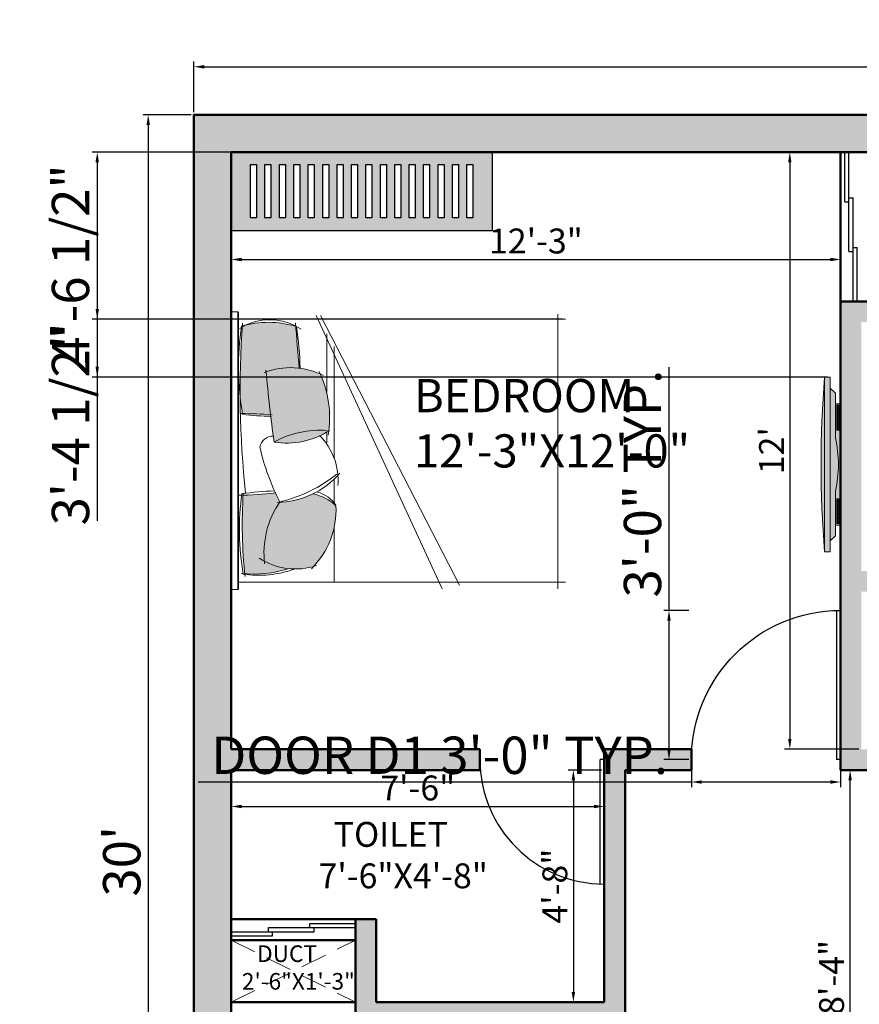
# Model space of a CAD drawing. Units: inches. Extents: x 3274 to 5176, y 1085 to 2172.
# Tile 13 of 16: x 4315 to 4518, y 1319 to 1556. Entities that reach past the tile are written whole.
import ezdxf

# ---------------------------------------------------------------- set-up
doc = ezdxf.new("R2010")
doc.units = ezdxf.units.IN
doc.linetypes.add('DASHED', pattern=[19.05, 12.7, -6.35])
for name, color, linetype, lineweight in [('0.10', 252, 'Continuous', 9), ('A-ANNO-DIMS', 2, 'Continuous', 18), ('A-AREA-IDEN', 3, 'Continuous', 25), ('A-DOOR', 4, 'Continuous', 25), ('A-EQPM', 8, 'Continuous', 18), ('A-FLOR-OPEN', 7, 'DASHED', 18), ('A-FLOR-PATT', 252, 'Continuous', 13), ('A-FURN', 8, 'Continuous', 18), ('A-GLAZ', 5, 'Continuous', 25), ('A-WALL', 7, 'Continuous', 50), ('A-WALL-PATT', 8, 'Continuous', 13), ('moveis', 254, 'Continuous', 5), ('parede', 7, 'Continuous', 30)]:
    doc.layers.add(name, color=color, linetype=linetype, lineweight=lineweight)
doc.layers.add('MESA', color=7, linetype='Continuous')
doc.styles.get("Standard").update_dxf_attribs({"font": 'arial.ttf'})
doc.dimstyles.new('ISO-25', dxfattribs={"dimtxt": 9, "dimasz": 2.5, "dimexe": 1.25, "dimexo": 0.625, "dimtad": 1, "dimdec": 1, "dimlunit": 3, "dimtxsty": 'Standard', "dimcen": 2.5, "dimclrd": 4, "dimclre": 4, "dimclrt": 1, "dimadec": 0, "dimazin": 0, "dimtfac": 1, "dimtdec": 1, "dimtmove": 0, "dimatfit": 3, "dimfxl": 1, "dimarcsym": 0})

# ---------------------------------------------------------------- blocks, each defined once
blk = doc.blocks.new('1')
for p, q in [((0, 36), (0, 0)), ((1, 36), (1, 0)), ((0, 0), (1, 0))]:
    blk.add_line(p, q)
blk.add_arc((0, 0), 36, 0, 90)
blk = doc.blocks.new('2')
for p, q in [((0, 30), (0, 0)), ((1, 30), (1, 0)), ((0, 0), (1, 0))]:
    blk.add_line(p, q)
blk.add_arc((0, 0), 30, 0, 90)
blk = doc.blocks.new('*D6')
at = {"layer": 'A-ANNO-DIMS', "color": 0, "lineweight": -2, "transparency": 16777216}
for p, q in [((4357.19, 1533.98), (4357.19, 1546.17)), ((4717.19, 1533.98), (4717.19, 1546.17)), ((4359.69, 1544.92), (4714.69, 1544.92))]:
    blk.add_line(p, q, dxfattribs=at)
at = {"layer": 'A-ANNO-DIMS', "color": 0, "transparency": 16777216}
for points in [[(4359.69, 1545.33), (4359.69, 1544.5), (4357.19, 1544.92)], [(4714.69, 1545.33), (4714.69, 1544.5), (4717.19, 1544.92)]]:
    blk.add_solid(points, dxfattribs=at)
at = {"layer": 'Defpoints', "color": 0, "transparency": 16777216}
for p in [(4717.19, 1544.92), (4357.19, 1533.35), (4717.19, 1533.35)]:
    blk.add_point(p, dxfattribs=at)
at = {"layer": 'A-ANNO-DIMS', "color": 0, "transparency": 16777216, "insert": (4537.19, 1550.14), "char_height": 9, "attachment_point": 5}
blk.add_mtext("30'", dxfattribs=at)
blk = doc.blocks.new('*D7')
at = {"layer": 'A-ANNO-DIMS', "color": 0, "lineweight": -2, "transparency": 16777216}
for p, q in [((4356.56, 1533.35), (4344.93, 1533.35)), ((4346.18, 1530.85), (4346.18, 1175.85)), ((4356.56, 1173.35), (4344.93, 1173.35))]:
    blk.add_line(p, q, dxfattribs=at)
at = {"layer": 'A-ANNO-DIMS', "color": 0, "transparency": 16777216}
for points in [[(4345.77, 1530.85), (4346.6, 1530.85), (4346.18, 1533.35)], [(4345.77, 1175.85), (4346.6, 1175.85), (4346.18, 1173.35)]]:
    blk.add_solid(points, dxfattribs=at)
at = {"layer": 'Defpoints', "color": 0, "transparency": 16777216}
for p in [(4357.19, 1533.35), (4346.18, 1173.35), (4357.19, 1173.35)]:
    blk.add_point(p, dxfattribs=at)
at = {"layer": 'A-ANNO-DIMS', "color": 0, "transparency": 16777216, "insert": (4340.96, 1353.35), "char_height": 9, "attachment_point": 5, "rotation": 90}
blk.add_mtext("30'", dxfattribs=at)
blk = doc.blocks.new('camita')
at = {"layer": '0.10'}
for p, q in [((-0.85, -0.045), (0.85, -0.045)), ((-0.805, -0.045), (-0.805, -2.0485)), ((0.805, -0.045), (0.805, -2.0485)), ((-0.8271, -0.521), (0.8464, -1.2932)), ((-0.8271, -0.5476), (0.8236, -1.3992)), ((-0.7161, -0.585), (-0.3554, -0.585)), ((-0.1136, -0.585), (-0.0485, -0.585)), ((-0.638, -0.63), (0.0434, -0.63)), ((0.1749, -0.63), (0.3179, -0.63)), ((0.4739, -0.63), (0.805, -0.63)), ((-0.8354, -2), (0.8464, -2))]:
    blk.add_line(p, q, dxfattribs=at)
blk.add_lwpolyline([(-0.85, -0.0405), (0.85, -0.0405), (0.85, 0), (-0.85, 0)], close=True, dxfattribs=at)
for centre, radius, start, end in [((-0.4574, -0.2364), 0.3443, 147.50996, 213.83359), ((-0.3639, -5.8457), 5.7909, 83.80731, 94.12107), ((-0.5104, -1.7232), 1.6781, 80.12554, 98.66187), ((2.3534, -0.0532), 2.5803, 180.10628, 184.38541), ((-1.4396, -0.0609), 1.7117, 352.92911, 0.39592), ((0.4863, -1.6286), 1.5781, 80.16015, 98.05996), ((-0.1997, -0.2266), 0.5864, 163.92635, 197.14087), ((-1.5443, -0.2452), 1.3333, 359.93941, 7.55329), ((1.5815, -0.2893), 1.3353, 170.38021, 178.99138), ((0.4524, -3.0675), 2.9996, 83.90257, 93.67595), ((0.0294, -0.1377), 0.7262, 342.58415, 6.00484), ((0.1326, -0.1696), 0.6307, 339.92303, 8.74334), ((-0.007, -0.258), 0.0828, 100.01798, 179.73597), ((-0.2931, -1.4378), 1.2903, 61.97485, 77.84351), ((0.3203, -0.3944), 0.4043, 341.45245, 33.45121), ((-0.0543, -0.3633), 0.4542, 159.30257, 206.50263), ((-1.3301, -9.6748), 9.4985, 82.27078, 84.93989), ((0.6265, -0.7518), 0.5508, 82.96906, 124.67388), ((0.4585, -0.5454), 0.5842, 151.04555, 184.14969), ((-0.5341, -0.3393), 0.4875, 327.26442, 9.0473), ((-0.1986, -0.2742), 0.5159, 310.73945, 359.05759), ((-0.5673, -0.0868), 0.9057, 321.69527, 346.46261), ((-1.8672, -14.986), 14.6323, 84.65974, 85.75157), ((-0.4598, 1.4861), 1.9092, 260.95299, 268.65169), ((-0.2002, 0.064), 0.6673, 244.78094, 279.06058), ((0.179, -0.272), 0.3828, 224.52836, 275.22287), ((0.4384, -0.4834), 0.1898, 193.68485, 236.70352), ((0.5707, -0.4317), 0.3145, 192.93877, 221.96363), ((0.3612, -0.133), 0.5096, 267.25889, 315.29965)]:
    blk.add_arc(centre, radius, start, end, dxfattribs=at)
blk = doc.blocks.new('Banco Lintz')
at = {"layer": 'MESA', "ltscale": 0.05}
h = blk.add_hatch(color=256, dxfattribs=at)
h.dxf.hatch_style = 1
h.set_gradient(color1=(138, 84, 66), color2=(0, 0, 0), one_color=1, name='INVCYLINDER')
h.paths.add_polyline_path([(0.48, 0), (0, 0), (0, -1.6), (0.48, -1.6)])
h.paths.add_polyline_path([(0.4034, -0.5091), (0.0766, -0.5091), (0.0766, -0.4724), (0.4034, -0.4724)], flags=16)
h.paths.add_polyline_path([(0.4034, -0.5608), (0.4034, -0.5974), (0.0766, -0.5974), (0.0766, -0.5608)], flags=16)
h.paths.add_polyline_path([(0.4034, -0.4207), (0.0766, -0.4207), (0.0766, -0.384), (0.4034, -0.384)], flags=16)
h.paths.add_polyline_path([(0.4034, -0.6491), (0.4034, -0.6858), (0.0766, -0.6858), (0.0766, -0.6491)], flags=16)
h.paths.add_polyline_path([(0.4034, -0.3323), (0.0766, -0.3323), (0.0766, -0.2957), (0.4034, -0.2957)], flags=16)
h.paths.add_polyline_path([(0.4034, -0.7375), (0.4034, -0.7741), (0.0766, -0.7741), (0.0766, -0.7375)], flags=16)
h.paths.add_polyline_path([(0.4034, -0.244), (0.0766, -0.244), (0.0766, -0.2073), (0.4034, -0.2073)], flags=16)
h.paths.add_polyline_path([(0.4034, -0.8259), (0.4034, -0.8625), (0.0766, -0.8625), (0.0766, -0.8259)], flags=16)
h.paths.add_polyline_path([(0.4034, -0.1556), (0.0766, -0.1556), (0.0766, -0.119), (0.4034, -0.119)], flags=16)
h.paths.add_polyline_path([(0.4034, -0.9142), (0.4034, -0.9509), (0.0766, -0.9509), (0.0766, -0.9142)], flags=16)
h.paths.add_polyline_path([(0.4034, -1.0026), (0.4034, -1.0392), (0.0766, -1.0392), (0.0766, -1.0026)], flags=16)
h.paths.add_polyline_path([(0.4034, -1.0909), (0.4034, -1.1276), (0.0766, -1.1276), (0.0766, -1.0909)], flags=16)
h.paths.add_polyline_path([(0.4034, -1.1793), (0.4034, -1.216), (0.0766, -1.216), (0.0766, -1.1793)], flags=16)
h.paths.add_polyline_path([(0.4034, -1.2677), (0.4034, -1.3043), (0.0766, -1.3043), (0.0766, -1.2677)], flags=16)
h.paths.add_polyline_path([(0.4034, -1.356), (0.4034, -1.3927), (0.0766, -1.3927), (0.0766, -1.356)], flags=16)
h.paths.add_polyline_path([(0.4034, -1.4444), (0.4034, -1.481), (0.0766, -1.481), (0.0766, -1.4444)], flags=16)
for points in [[(0, -1.6), (0.48, -1.6), (0.48, 0), (0, 0)], [(0.0766, -0.119), (0.4034, -0.119), (0.4034, -0.1556), (0.0766, -0.1556)], [(0.0766, -0.2073), (0.4034, -0.2073), (0.4034, -0.244), (0.0766, -0.244)], [(0.0766, -0.2957), (0.4034, -0.2957), (0.4034, -0.3323), (0.0766, -0.3323)], [(0.0766, -0.384), (0.4034, -0.384), (0.4034, -0.4207), (0.0766, -0.4207)], [(0.0766, -0.4724), (0.4034, -0.4724), (0.4034, -0.5091), (0.0766, -0.5091)], [(0.0766, -0.5608), (0.4034, -0.5608), (0.4034, -0.5974), (0.0766, -0.5974)], [(0.0766, -0.6491), (0.4034, -0.6491), (0.4034, -0.6858), (0.0766, -0.6858)], [(0.0766, -0.7375), (0.4034, -0.7375), (0.4034, -0.7741), (0.0766, -0.7741)], [(0.0766, -0.8259), (0.4034, -0.8259), (0.4034, -0.8625), (0.0766, -0.8625)], [(0.0766, -0.9142), (0.4034, -0.9142), (0.4034, -0.9509), (0.0766, -0.9509)], [(0.0766, -1.0026), (0.4034, -1.0026), (0.4034, -1.0392), (0.0766, -1.0392)], [(0.0766, -1.0909), (0.4034, -1.0909), (0.4034, -1.1276), (0.0766, -1.1276)], [(0.0766, -1.1793), (0.4034, -1.1793), (0.4034, -1.216), (0.0766, -1.216)], [(0.0766, -1.2677), (0.4034, -1.2677), (0.4034, -1.3043), (0.0766, -1.3043)], [(0.0766, -1.356), (0.4034, -1.356), (0.4034, -1.3927), (0.0766, -1.3927)], [(0.0766, -1.4444), (0.4034, -1.4444), (0.4034, -1.481), (0.0766, -1.481)]]:
    blk.add_lwpolyline(points, close=True, dxfattribs=at)
blk = doc.blocks.new('PLASMA 2')
at = {"layer": 'moveis', "ltscale": 0.08}
h = blk.add_hatch(dxfattribs=at)
h.set_pattern_fill('_USER,_O', color=256, scale=0.008, double=1, pattern_type=0)
h.set_pattern_definition([(360, (-4.134502, -6.848382), (0, 0.008), []), (90, (-4.134502, -6.848382), (-0.008, 0), [])])
h.paths.add_polyline_path([(-0.2099, -0.0965), (-0.3623, -0.0965), (-0.3623, -0.1111), (-0.2099, -0.1111)])
h = blk.add_hatch(dxfattribs=at)
h.set_pattern_fill('_USER,_O', color=256, scale=0.008, double=1, pattern_type=0)
h.set_pattern_definition([(180, (4.134502, -6.848382), (0, 0.008), []), (90, (4.134502, -6.848382), (0.008, 0), [])])
h.paths.add_polyline_path([(0.2099, -0.0965), (0.3623, -0.0965), (0.3623, -0.1111), (0.2099, -0.1111)])
at = {"layer": 'parede', "ltscale": 0.08}
h = blk.add_hatch(color=256, dxfattribs=at)
h.dxf.hatch_style = 1
h.set_gradient(color1=(131, 136, 145), one_color=1, tint=1, name='CURVED')
h.paths.add_polyline_path([(-0.535, -0.0215), (0.535, -0.0215, 0.040195)])
h = blk.add_hatch(color=256, dxfattribs=at)
h.dxf.hatch_style = 1
h.set_gradient(color1=(131, 136, 145), color2=(0, 0, 0), one_color=1, name='CURVED')
h.paths.add_polyline_path([(0.535, -0.0215), (-0.535, -0.0215), (-0.535, -0.0553), (0.535, -0.0553)])
h = blk.add_hatch(color=256, dxfattribs=at)
h.dxf.hatch_style = 1
h.set_gradient(color1=(131, 136, 145), one_color=1, tint=1, name='CYLINDER')
h.paths.add_polyline_path([(0.4673, -0.0553), (-0.4673, -0.0553), (-0.4363, -0.0876), (-0.1636, -0.0876, 0.114423), (0.1636, -0.0876), (0.4363, -0.0876)])
h = blk.add_hatch(color=256, dxfattribs=at)
h.dxf.hatch_style = 1
h.set_gradient(color1=(131, 136, 145), color2=(0, 0, 0), one_color=1, name='CURVED')
h.paths.add_polyline_path([(0.3724, -0.0876), (0.1636, -0.0876, -0.114423), (-0.1636, -0.0876), (-0.3724, -0.0876), (-0.3724, -0.12), (0.3724, -0.12)])
h.paths.add_polyline_path([(-0.2099, -0.1111), (-0.3623, -0.1111), (-0.3623, -0.0965), (-0.2099, -0.0965)], flags=16)
h.paths.add_polyline_path([(0.2099, -0.1111), (0.2099, -0.0965), (0.3623, -0.0965), (0.3623, -0.1111)], flags=16)
at = {"layer": 'moveis', "ltscale": 0.08}
for p, q in [((-0.535, -0.0215), (-0.535, -0.0553)), ((-0.535, -0.0215), (0.535, -0.0215)), ((0.535, -0.0553), (-0.535, -0.0553)), ((-0.4673, -0.0553), (-0.4363, -0.0876)), ((0.4673, -0.0553), (0.4363, -0.0876)), ((0.535, -0.0553), (0.535, -0.0215)), ((-0.4363, -0.0876), (-0.1636, -0.0876)), ((-0.3724, -0.0876), (-0.3724, -0.12)), ((-0.3724, -0.12), (0.3724, -0.12)), ((0.1636, -0.0876), (0.4363, -0.0876)), ((0.3724, -0.0876), (0.3724, -0.12))]:
    blk.add_line(p, q, dxfattribs=at)
for points in [[(-0.3623, -0.0965), (-0.2099, -0.0965), (-0.2099, -0.1111), (-0.3623, -0.1111)], [(0.3623, -0.0965), (0.2099, -0.0965), (0.2099, -0.1111), (0.3623, -0.1111)]]:
    blk.add_lwpolyline(points, close=True, dxfattribs=at)
for centre, radius, start, end in [((0, -6.6658), 6.6658, 85.39647, 94.60353), ((0, 0.6178), 0.7242, 256.94486, 283.05514)]:
    blk.add_arc(centre, radius, start, end, dxfattribs=at)
blk = doc.blocks.new('*D69')
at = {"layer": 'A-ANNO-DIMS', "color": 0, "lineweight": -2, "transparency": 16777216}
for p, q in [((4366.19, 1523.73), (4366.19, 1497.19)), ((4513.19, 1523.73), (4513.19, 1497.19)), ((4368.69, 1498.44), (4510.69, 1498.44))]:
    blk.add_line(p, q, dxfattribs=at)
at = {"layer": 'A-ANNO-DIMS', "color": 0, "transparency": 16777216}
for points in [[(4368.69, 1498.86), (4368.69, 1498.03), (4366.19, 1498.44)], [(4510.69, 1498.86), (4510.69, 1498.03), (4513.19, 1498.44)]]:
    blk.add_solid(points, dxfattribs=at)
at = {"layer": 'Defpoints', "color": 0, "transparency": 16777216}
for p in [(4366.19, 1524.35), (4513.19, 1524.35), (4513.19, 1498.44)]:
    blk.add_point(p, dxfattribs=at)
at = {"layer": 'A-ANNO-DIMS', "color": 0, "transparency": 16777216, "insert": (4439.69, 1502.13), "char_height": 6, "attachment_point": 5}
blk.add_mtext('12\'-3"', dxfattribs=at)
blk = doc.blocks.new('*D70')
at = {"layer": 'A-ANNO-DIMS', "color": 0, "lineweight": -2, "transparency": 16777216}
for p, q in [((4512.56, 1524.35), (4499.67, 1524.35)), ((4500.92, 1521.85), (4500.92, 1382.85)), ((4517.56, 1380.35), (4499.67, 1380.35))]:
    blk.add_line(p, q, dxfattribs=at)
at = {"layer": 'A-ANNO-DIMS', "color": 0, "transparency": 16777216}
for points in [[(4500.51, 1521.85), (4501.34, 1521.85), (4500.92, 1524.35)], [(4500.51, 1382.85), (4501.34, 1382.85), (4500.92, 1380.35)]]:
    blk.add_solid(points, dxfattribs=at)
at = {"layer": 'Defpoints', "color": 0, "transparency": 16777216}
for p in [(4513.19, 1524.35), (4500.92, 1380.35), (4518.19, 1380.35)]:
    blk.add_point(p, dxfattribs=at)
at = {"layer": 'A-ANNO-DIMS', "color": 0, "transparency": 16777216, "insert": (4497.29, 1452.35), "char_height": 6, "attachment_point": 5, "rotation": 90}
blk.add_mtext("12'", dxfattribs=at)
blk = doc.blocks.new('*D71')
at = {"layer": 'A-ANNO-DIMS', "color": 0, "lineweight": -2, "transparency": 16777216}
for p, q in [((4366.19, 1374.73), (4366.19, 1365.31)), ((4456.19, 1374.73), (4456.19, 1365.31)), ((4368.69, 1366.56), (4453.69, 1366.56))]:
    blk.add_line(p, q, dxfattribs=at)
at = {"layer": 'A-ANNO-DIMS', "color": 0, "transparency": 16777216}
for points in [[(4368.69, 1366.97), (4368.69, 1366.14), (4366.19, 1366.56)], [(4453.69, 1366.97), (4453.69, 1366.14), (4456.19, 1366.56)]]:
    blk.add_solid(points, dxfattribs=at)
at = {"layer": 'Defpoints', "color": 0, "transparency": 16777216}
for p in [(4366.19, 1375.35), (4456.19, 1375.35), (4456.19, 1366.56)]:
    blk.add_point(p, dxfattribs=at)
at = {"layer": 'A-ANNO-DIMS', "color": 0, "transparency": 16777216, "insert": (4411.19, 1370.24), "char_height": 6, "attachment_point": 5}
blk.add_mtext('7\'-6"', dxfattribs=at)
blk = doc.blocks.new('*D72')
at = {"layer": 'A-ANNO-DIMS', "color": 0, "lineweight": -2, "transparency": 16777216}
for p, q in [((4455.56, 1375.35), (4447.47, 1375.35)), ((4448.72, 1372.85), (4448.72, 1321.85)), ((4455.56, 1319.35), (4447.47, 1319.35))]:
    blk.add_line(p, q, dxfattribs=at)
at = {"layer": 'A-ANNO-DIMS', "color": 0, "transparency": 16777216}
for points in [[(4448.3, 1372.85), (4449.14, 1372.85), (4448.72, 1375.35)], [(4448.3, 1321.85), (4449.14, 1321.85), (4448.72, 1319.35)]]:
    blk.add_solid(points, dxfattribs=at)
at = {"layer": 'Defpoints', "color": 0, "transparency": 16777216}
for p in [(4456.19, 1375.35), (4448.72, 1319.35), (4456.19, 1319.35)]:
    blk.add_point(p, dxfattribs=at)
at = {"layer": 'A-ANNO-DIMS', "color": 0, "transparency": 16777216, "insert": (4445.03, 1347.35), "char_height": 6, "attachment_point": 5, "rotation": 90}
blk.add_mtext('4\'-8"', dxfattribs=at)
blk = doc.blocks.new('*D82')
at = {"layer": 'A-ANNO-DIMS', "color": 0, "lineweight": -2, "transparency": 16777216}
for p, q in [((4513.81, 1375.35), (4516.72, 1375.35)), ((4515.47, 1277.85), (4515.47, 1372.85)), ((4513.81, 1275.35), (4516.72, 1275.35))]:
    blk.add_line(p, q, dxfattribs=at)
at = {"layer": 'A-ANNO-DIMS', "color": 0, "transparency": 16777216}
for points in [[(4515.05, 1372.85), (4515.88, 1372.85), (4515.47, 1375.35)], [(4515.05, 1277.85), (4515.88, 1277.85), (4515.47, 1275.35)]]:
    blk.add_solid(points, dxfattribs=at)
at = {"layer": 'Defpoints', "color": 0, "transparency": 16777216}
for p in [(4513.19, 1375.35), (4515.47, 1375.35), (4513.19, 1275.35)]:
    blk.add_point(p, dxfattribs=at)
at = {"layer": 'A-ANNO-DIMS', "color": 0, "transparency": 16777216, "insert": (4511.78, 1325.35), "char_height": 6, "attachment_point": 5, "rotation": 90}
blk.add_mtext('8\'-4"', dxfattribs=at)
blk = doc.blocks.new('WIN-30')
for p, q in [((4385.19, 1318.35), (4396.19, 1318.35)), ((4385.19, 1317.35), (4385.19, 1318.35)), ((4366.19, 1316.35), (4386.19, 1316.35)), ((4366.19, 1315.35), (4376.19, 1315.35)), ((4375.19, 1317.35), (4396.19, 1317.35)), ((4375.19, 1316.35), (4375.19, 1317.35)), ((4376.19, 1315.35), (4376.19, 1316.35)), ((4386.19, 1316.35), (4386.19, 1317.35))]:
    blk.add_line(p, q)
blk = doc.blocks.new('WIN-36')
for p, q in [((4514.19, 1512.35), (4514.19, 1524.35)), ((4515.19, 1500.35), (4515.19, 1524.35)), ((4514.19, 1512.35), (4515.19, 1512.35)), ((4515.19, 1513.35), (4516.19, 1513.35)), ((4516.19, 1488.35), (4516.19, 1513.35)), ((4516.19, 1501.35), (4517.19, 1501.35)), ((4517.19, 1488.35), (4517.19, 1501.35)), ((4515.19, 1500.35), (4516.19, 1500.35))]:
    blk.add_line(p, q)
blk = doc.blocks.new('*D114')
at = {"layer": 'A-ANNO-DIMS', "color": 4, "lineweight": -2, "transparency": 16777216}
for p, q in [((4477.19, 1377.23), (4477.19, 1371.2)), ((4513.19, 1377.23), (4513.19, 1371.2)), ((4477.19, 1372.45), (4358.25, 1372.45)), ((4510.69, 1372.45), (4479.69, 1372.45))]:
    blk.add_line(p, q, dxfattribs=at)
at = {"layer": 'A-ANNO-DIMS', "color": 4, "transparency": 16777216}
for points in [[(4479.69, 1372.87), (4479.69, 1372.04), (4477.19, 1372.45)], [(4510.69, 1372.87), (4510.69, 1372.04), (4513.19, 1372.45)]]:
    blk.add_solid(points, dxfattribs=at)
at = {"layer": 'Defpoints', "color": 0, "transparency": 16777216}
for p in [(4477.19, 1377.85), (4513.19, 1377.85), (4477.19, 1372.45)]:
    blk.add_point(p, dxfattribs=at)
at = {"layer": 'A-ANNO-DIMS', "color": 1, "transparency": 16777216, "insert": (4416.47, 1377.74), "char_height": 9, "attachment_point": 5}
blk.add_mtext('DOOR D1 3\'-0" TYP.', dxfattribs=at)
blk = doc.blocks.new('*D115')
at = {"layer": 'A-ANNO-DIMS', "color": 4, "lineweight": -2, "transparency": 16777216}
for p, q in [((4471.79, 1413.85), (4471.79, 1472.46)), ((4476.56, 1413.85), (4470.54, 1413.85)), ((4471.79, 1380.35), (4471.79, 1411.35)), ((4476.56, 1377.85), (4470.54, 1377.85))]:
    blk.add_line(p, q, dxfattribs=at)
at = {"layer": 'A-ANNO-DIMS', "color": 4, "transparency": 16777216}
for points in [[(4471.37, 1411.35), (4472.2, 1411.35), (4471.79, 1413.85)], [(4471.37, 1380.35), (4472.2, 1380.35), (4471.79, 1377.85)]]:
    blk.add_solid(points, dxfattribs=at)
at = {"layer": 'Defpoints', "color": 0, "transparency": 16777216}
for p in [(4471.79, 1413.85), (4477.19, 1413.85), (4477.19, 1377.85)]:
    blk.add_point(p, dxfattribs=at)
at = {"layer": 'A-ANNO-DIMS', "color": 1, "transparency": 16777216, "insert": (4466.56, 1444.41), "char_height": 9, "attachment_point": 5, "rotation": 90}
blk.add_mtext('3\'-0" TYP.', dxfattribs=at)
blk = doc.blocks.new('*D156')
at = {"layer": 'A-ANNO-DIMS', "color": 4, "lineweight": -2, "transparency": 16777216}
for p, q in [((4365.56, 1524.35), (4332.64, 1524.35)), ((4333.89, 1521.85), (4333.89, 1486.55)), ((4446.22, 1484.05), (4332.64, 1484.05)), ((4333.89, 1484.05), (4333.89, 1435.41))]:
    blk.add_line(p, q, dxfattribs=at)
at = {"layer": 'A-ANNO-DIMS', "color": 4, "transparency": 16777216}
for points in [[(4333.47, 1521.85), (4334.3, 1521.85), (4333.89, 1524.35)], [(4333.47, 1486.55), (4334.3, 1486.55), (4333.89, 1484.05)]]:
    blk.add_solid(points, dxfattribs=at)
at = {"layer": 'Defpoints', "color": 0, "transparency": 16777216}
for p in [(4366.19, 1524.35), (4333.89, 1484.05), (4446.85, 1484.05)]:
    blk.add_point(p, dxfattribs=at)
at = {"layer": 'A-ANNO-DIMS', "color": 1, "transparency": 16777216, "insert": (4328.61, 1458.48), "char_height": 9, "attachment_point": 5, "rotation": 90}
blk.add_mtext('3\'-4 1/2"', dxfattribs=at)
blk = doc.blocks.new('*D158')
at = {"layer": 'A-ANNO-DIMS', "color": 4, "lineweight": -2, "transparency": 16777216}
for p, q in [((4512.56, 1524.35), (4332.64, 1524.35)), ((4333.89, 1521.85), (4333.89, 1472.58)), ((4510.01, 1470.08), (4332.64, 1470.08))]:
    blk.add_line(p, q, dxfattribs=at)
at = {"layer": 'A-ANNO-DIMS', "color": 4, "transparency": 16777216}
for points in [[(4333.47, 1521.85), (4334.3, 1521.85), (4333.89, 1524.35)], [(4333.47, 1472.58), (4334.3, 1472.58), (4333.89, 1470.08)]]:
    blk.add_solid(points, dxfattribs=at)
at = {"layer": 'Defpoints', "color": 0, "transparency": 16777216}
for p in [(4513.19, 1524.35), (4333.89, 1470.08), (4510.64, 1470.08)]:
    blk.add_point(p, dxfattribs=at)
at = {"layer": 'A-ANNO-DIMS', "color": 1, "transparency": 16777216, "insert": (4328.61, 1497.22), "char_height": 9, "attachment_point": 5, "rotation": 90}
blk.add_mtext('4\'-6 1/2"', dxfattribs=at)

msp = doc.modelspace()

# ---------------------------------------------------------------- hatches: boundary and pattern name
at = {"layer": 'A-FLOR-PATT'}
h = msp.add_hatch(color=256, dxfattribs=at)
h.dxf.hatch_style = 1
h.paths.add_polyline_path([(4381.76, 1482.32, 0.131047), (4369.87, 1482.7, 0.020657), (4368.87, 1482.2, 0.01851), (4368.35, 1465.33, 0.015442), (4368.91, 1461.29, -0.016701), (4375.69, 1461.02, -0.006967), (4374.62, 1471.38, -0.113891), (4382.62, 1472.25, -0.004387)])
h.paths.add_polyline_path([(4377.95, 1440.02, -0.011742), (4376.88, 1442.15, -0.029051), (4369.07, 1441.64, 0.040212), (4369.46, 1422.68, 0.094792), (4380.13, 1423.9, -0.098488), (4374.19, 1425.71, -0.175864)])
h.paths.add_polyline_path([(4387.7, 1470.86, 0.189536), (4374.62, 1471.38, 0.011408), (4376.53, 1454.43, 0.181694), (4389.76, 1457.13, 0.134508)])
h.paths.add_polyline_path([(4391.47, 1439.09, 0.127326), (4385.96, 1441.95, -0.104045), (4377.86, 1439.88, 0.173835), (4374.19, 1425.71, 0.194952), (4386.08, 1424.43, 0.202559)])
at = {"layer": 'A-WALL-PATT'}
h = msp.add_hatch(color=256, dxfattribs=at)
h.dxf.hatch_style = 1
h.paths.add_polyline_path([(4717.19, 1533.35), (4357.19, 1533.35), (4357.19, 1173.35), (4390.19, 1173.35), (4390.19, 1182.35), (4366.19, 1182.35), (4366.19, 1266.35), (4426.19, 1266.35), (4426.19, 1271.35), (4366.19, 1271.35), (4366.19, 1375.35), (4426.19, 1375.35), (4426.19, 1380.35), (4366.19, 1380.35), (4366.19, 1524.35), (4708.19, 1524.35), (4708.19, 1380.35), (4578.19, 1380.35), (4578.19, 1375.35), (4708.19, 1375.35), (4708.19, 1275.35), (4640.19, 1275.35), (4640.19, 1266.35), (4708.19, 1266.35), (4708.19, 1182.35), (4666.19, 1182.35), (4666.19, 1173.35), (4717.19, 1173.35)])
h.paths.add_polyline_path([(4461.19, 1375.35), (4477.19, 1375.35), (4477.19, 1380.35), (4456.19, 1380.35), (4456.19, 1319.35), (4401.19, 1319.35), (4401.19, 1339.35), (4396.19, 1339.35), (4396.19, 1314.35), (4456.19, 1314.35), (4456.19, 1266.35), (4477.19, 1266.35), (4477.19, 1271.35), (4461.19, 1271.35)], flags=17)
h.paths.add_polyline_path([(4518.19, 1483.35), (4536.19, 1483.35), (4536.19, 1488.35), (4513.19, 1488.35), (4513.19, 1375.35), (4536.19, 1375.35), (4536.19, 1380.35), (4518.19, 1380.35), (4518.19, 1418.35), (4548.19, 1418.35), (4548.19, 1423.35), (4518.19, 1423.35)], flags=17)
h.paths.add_polyline_path([(4583.19, 1488.35), (4560.19, 1488.35), (4560.19, 1483.35), (4578.19, 1483.35), (4578.19, 1416.35), (4583.19, 1416.35)], flags=17)
h.paths.add_polyline_path([(4518.19, 1266.35), (4523.19, 1266.35), (4523.19, 1275.35), (4513.19, 1275.35), (4513.19, 1182.35), (4462.19, 1182.35), (4462.19, 1173.35), (4518.19, 1173.35)], flags=17)
h.paths.add_polyline_path([(4580.19, 1275.35), (4571.19, 1275.35), (4571.19, 1270.85), (4571.19, 1266.35), (4580.19, 1266.35)], flags=17)
h.paths.add_polyline_path([(4594.19, 1182.35), (4578.19, 1182.35), (4578.19, 1173.35), (4594.19, 1173.35)], flags=17)
h.paths.add_polyline_path([(4573.24, 1316.29), (4647.44, 1316.29), (4647.44, 1346.14), (4573.24, 1346.14)], flags=25)
h.paths.add_polyline_path([(4529.43, 1453), (4568.61, 1453), (4568.61, 1475.39), (4529.43, 1475.39)], flags=25)
h.paths.add_polyline_path([(4619, 1443.76), (4687.39, 1443.76), (4687.39, 1473.61), (4619, 1473.61)], flags=25)
h.paths.add_polyline_path([(4527.67, 1497.04), (4569.64, 1497.04), (4569.64, 1519.43), (4527.67, 1519.43)], flags=25)
h.paths.add_polyline_path([(4407.08, 1443.76), (4475.47, 1443.76), (4475.47, 1473.61), (4407.08, 1473.61)], flags=25)

# ---------------------------------------------------------------- linework, layer by layer
at = {"layer": 'A-FLOR-OPEN', "ltscale": 0.5}
for p, q in [((4366.19, 1334.35), (4396.19, 1319.35)), ((4366.19, 1319.35), (4396.19, 1334.35))]:
    msp.add_line(p, q, dxfattribs=at)
at = {"layer": 'A-WALL'}
for p, q in [((4366.19, 1524.35), (4708.19, 1524.35)), ((4366.19, 1380.35), (4366.19, 1524.35)), ((4513.19, 1375.35), (4513.19, 1524.35)), ((4513.19, 1488.35), (4583.19, 1488.35)), ((4366.19, 1380.35), (4426.19, 1380.35)), ((4426.19, 1375.35), (4426.19, 1380.35)), ((4456.19, 1319.35), (4456.19, 1380.35)), ((4456.19, 1380.35), (4477.19, 1380.35)), ((4477.19, 1375.35), (4477.19, 1380.35)), ((4366.19, 1375.35), (4426.19, 1375.35)), ((4366.19, 1271.35), (4366.19, 1375.35)), ((4461.19, 1271.35), (4461.19, 1375.35)), ((4461.19, 1375.35), (4477.19, 1375.35)), ((4513.19, 1375.35), (4536.19, 1375.35)), ((4366.19, 1339.35), (4401.19, 1339.35)), ((4396.19, 1314.35), (4396.19, 1339.35)), ((4401.19, 1319.35), (4401.19, 1339.35)), ((4366.19, 1334.35), (4396.19, 1334.35)), ((4366.19, 1319.35), (4396.19, 1319.35)), ((4401.19, 1319.35), (4456.19, 1319.35))]:
    msp.add_line(p, q, dxfattribs=at)
msp.add_lwpolyline([(4518.19, 1173.35), (4357.19, 1173.35), (4357.19, 1533.35), (4717.19, 1533.35), (4717.19, 1173.35), (4578.19, 1173.35)], dxfattribs=at)

# ---------------------------------------------------------------- block references
at = {"layer": 'A-DOOR', "xscale": -1}
msp.add_blockref('1', (4513.19, 1377.85), dxfattribs=at)
at = {"layer": 'A-DOOR', "rotation": 180}
msp.add_blockref('2', (4456.19, 1377.85), dxfattribs=at)
at = {"layer": 'A-EQPM', "xscale": 39.37, "yscale": 39.37, "zscale": 39.37, "rotation": 90}
msp.add_blockref('PLASMA 2', (4508.46, 1449.02), dxfattribs=at)
at = {"layer": 'A-FURN'}
for name, p, xscale, yscale, zscale, rotation in [('Banco Lintz', (4429.18, 1524.35), 39.37, 39.37, 39.37, 270), ('camita', (4366.19, 1452.35), -39.375, 39.375, 39.375, 90)]:
    msp.add_blockref(name, p, dxfattribs=dict(at, xscale=xscale, yscale=yscale, zscale=zscale, rotation=rotation))
at = {"layer": 'A-GLAZ'}
for name, p in [('WIN-36', (0, 0)), ('WIN-30', (0, 20))]:
    msp.add_blockref(name, p, dxfattribs=at)

# ---------------------------------------------------------------- texts
at = {"layer": 'A-AREA-IDEN', "attachment_point": 1}
for s, heights, insert, char_height in [('BEDROOM\\P12\'-3"X12\'-0"', [0], (4410.29, 1469.63), 8), ('  TOILET\\P7\'-6"X4\'-8"', [16.24], (4387.26, 1362.83), 6), ('   DUCT\\P2\'-6"X1\'-3"', [16.24], (4368.78, 1333.06), 4)]:
    msp.add_mtext_dynamic_manual_height_columns(s, width=58.0121, gutter_width=30, heights=heights, dxfattribs=dict(at, insert=insert, char_height=char_height))

# ---------------------------------------------------------------- dimensions: what is measured, and where the dimension line sits
at = {"layer": 'A-ANNO-DIMS'}
for base, p1, p2, override, picture, middle in [((4717.19, 1544.92), (4357.19, 1533.35), (4717.19, 1533.35), {"dimclrd": 0, "dimclre": 0, "dimclrt": 0}, '*D6', (4537.19, 1550.14)), ((4513.19, 1498.44), (4366.19, 1524.35), (4513.19, 1524.35), {"dimtxt": 6, "dimclrd": 0, "dimclre": 0, "dimclrt": 0}, '*D69', (4439.69, 1502.13)), ((4456.19, 1366.56), (4366.19, 1375.35), (4456.19, 1375.35), {"dimtxt": 6, "dimclrd": 0, "dimclre": 0, "dimclrt": 0}, '*D71', (4411.19, 1370.24))]:
    dim = msp.add_linear_dim(base=base, p1=p1, p2=p2, dimstyle='ISO-25', override=override, dxfattribs=at)
    dim.commit()
    dim.dimension.update_dxf_attribs({"geometry": picture, "text_midpoint": middle})
for base, p1, p2, override, picture, middle in [((4346.18, 1173.35), (4357.19, 1533.35), (4357.19, 1173.35), {"dimclrd": 0, "dimclre": 0, "dimclrt": 0}, '*D7', (4340.96, 1353.35)), ((4333.89, 1484.05), (4366.19, 1524.35), (4446.85, 1484.05), {"dimdec": 1, "dimlfac": 1, "dimrnd": 0, "dimzin": 1, "dimdsep": 46, "dimlunit": 4, "dimfrac": 2}, '*D156', (4328.61, 1458.48)), ((4333.89, 1470.08), (4513.19, 1524.35), (4510.64, 1470.08), {"dimdec": 1, "dimlfac": 1, "dimrnd": 0, "dimzin": 1, "dimdsep": 46, "dimlunit": 4, "dimfrac": 2}, '*D158', (4328.61, 1497.22)), ((4500.92, 1380.35), (4513.19, 1524.35), (4518.19, 1380.35), {"dimtxt": 6, "dimclrd": 0, "dimclre": 0, "dimclrt": 0}, '*D70', (4497.29, 1452.35)), ((4448.72, 1319.35), (4456.19, 1375.35), (4456.19, 1319.35), {"dimtxt": 6, "dimclrd": 0, "dimclre": 0, "dimclrt": 0}, '*D72', (4445.03, 1347.35)), ((4515.47, 1375.35), (4513.19, 1275.35), (4513.19, 1375.35), {"dimtxt": 6, "dimclrd": 0, "dimclre": 0, "dimclrt": 0}, '*D82', (4511.78, 1325.35))]:
    dim = msp.add_linear_dim(base=base, p1=p1, p2=p2, angle=90, dimstyle='ISO-25', override=override, dxfattribs=at)
    dim.commit()
    dim.dimension.update_dxf_attribs({"geometry": picture, "text_midpoint": middle})
for base, p1, p2, angle, text, picture, middle in [((4471.79, 1413.85), (4477.19, 1377.85), (4477.19, 1413.85), 90, '<> TYP.', '*D115', (4466.56, 1444.41)), ((4477.19, 1372.45), (4513.19, 1377.85), (4477.19, 1377.85), 180, 'DOOR D1 <> TYP.', '*D114', (4416.47, 1377.74))]:
    dim = msp.add_linear_dim(base=base, p1=p1, p2=p2, angle=angle, text=text, dimstyle='ISO-25', override={"dimdec": 1, "dimrnd": 0, "dimzin": 1, "dimlunit": 4, "dimfrac": 2}, dxfattribs=at)
    dim.commit()
    dim.dimension.update_dxf_attribs({"geometry": picture, "text_midpoint": middle})

doc.saveas('drawing.dxf')
